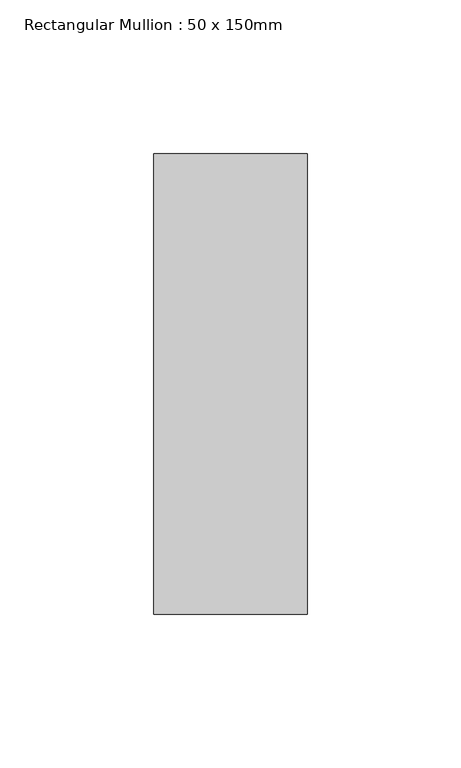
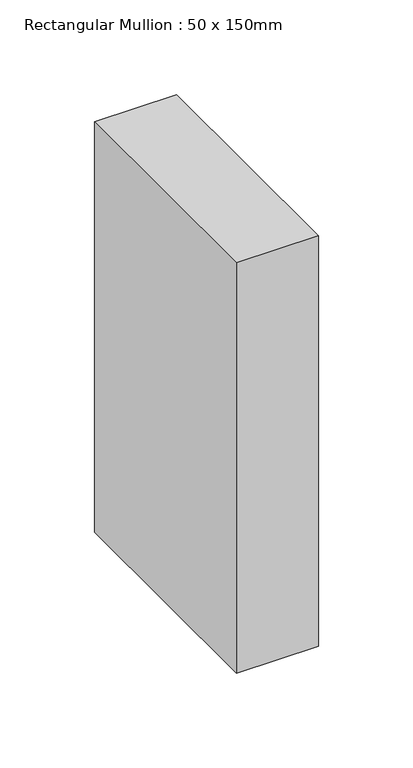
"""IFC4 building model written with IfcOpenShell, lengths in millimetres: member geometry, Rectangular Mullion : 50 x 150mm."""

from ifc_helpers import new_model, si_unit, frame, origin, place, context, project, spatial, polyline, outline, extrude, source, transform, mapped, element, save


def rectangular_mullion_50_x_150mm_987ee5f5(model_context):
    return source(origin(), model_context, "Body", "SweptSolid", [
        extrude(outline(polyline([(0.0, 75.0), (0.0, -75.0), (-50.0, -75.0), (-50.0, 75.0), (0.0, 75.0)])), frame((0.0, 0.0, -264.7981649), z_axis=(0.0, 0.0, 1.0), x_axis=(1.0, 0.0, 0.0)), (0.0, 0.0, 1.0), 264.7981649),
    ])


if __name__ == "__main__":
    model = new_model("IFC4")
    model_context = context("Model", 3, world=origin())
    ifc_project = project(units=[si_unit("LENGTHUNIT", "METRE", prefix="MILLI")], contexts=[model_context])
    site = spatial("IfcSite", under=ifc_project)
    building = spatial("IfcBuilding", under=site)
    placement = place(None, origin())
    rectangular_mullion_50_x_150mm_shape = rectangular_mullion_50_x_150mm_987ee5f5(model_context)
    element("IfcMember", 1, ObjectType="Rectangular Mullion : 50 x 150mm", at=placement, inside=building, context=model_context, shape_type="MappedRepresentation", body=[
        mapped(rectangular_mullion_50_x_150mm_shape, transform((0.0, 0.0, 0.0), x_axis=(1.0, 0.0, 0.0), y_axis=(0.0, 1.0, 0.0), z_axis=(0.0, 0.0, 1.0))),
    ])
    save(model, "model.ifc")

# Revit data of these elements
# Type "Rectangular Mullion : 50 x 150mm"
#   built-in parameter 1007304 = 0.492126 (stored number, unit not read)
#   built-in parameter 1007301 = 0.082021 (stored number, unit not read)
#   built-in parameter 1007300 = 0.082021 (stored number, unit not read)
# Element 1 (IfcMember, "Rectangular Mullion : 50 x 150mm")
#   Materials on its faces: "Aluminium"
# Materials
#   "Aluminium": class "Metal", colour RGB 247 247 247, transparency 0, Description = "Aluminium 6061", Cost = 0
